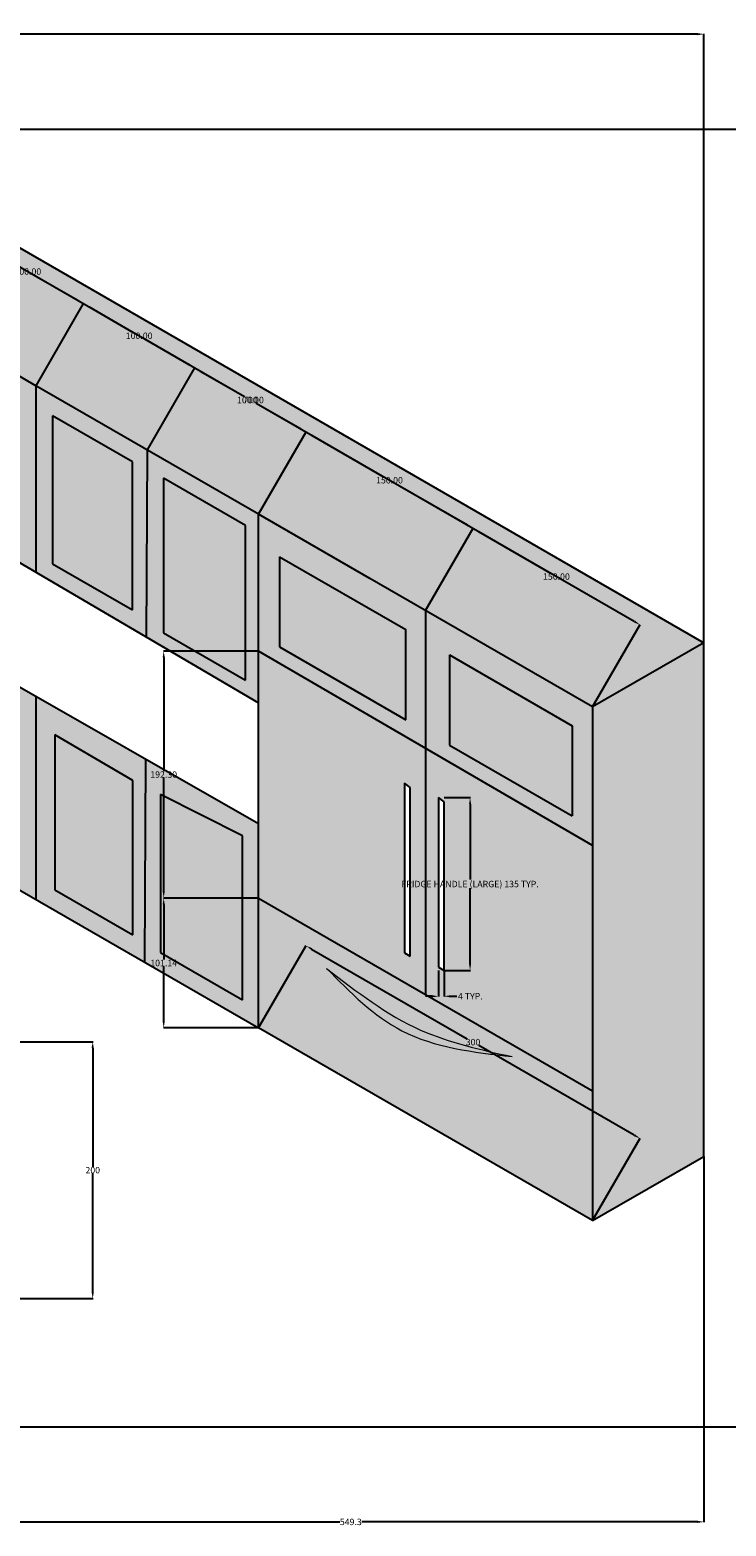
# Model space of a CAD drawing. Units: centimetres. Extents: x -744 to 1642, y 210 to 1375.
# Tile 4 of 8: x 288 to 830, y 210 to 1375. Entities that reach past the tile are written whole.
import ezdxf

# ---------------------------------------------------------------- set-up
doc = ezdxf.new("R2010")
doc.units = ezdxf.units.CM
doc.header["$MEASUREMENT"] = 0
for name, color, linetype, lineweight in [('A-ANNO-DIMS', 2, 'Continuous', 18), ('A-EQPM', 8, 'Continuous', 18), ('A-EQPM-PATT', 9, 'Continuous', 13), ('A-FURN', 7, 'Continuous', 25), ('A-FURN-PATT', 30, 'Continuous', 13), ('A-WALL-PATT', 61, 'Continuous', 13)]:
    doc.layers.add(name, color=color, linetype=linetype, lineweight=lineweight)
doc.styles.get("Standard").update_dxf_attribs({"font": 'arial.ttf'})
doc.dimstyles.get("Standard").update_dxf_attribs({"dimtxt": 5, "dimasz": 5, "dimexe": 0.18, "dimexo": 0.0625, "dimgap": 0.09, "dimtad": 0, "dimtih": 1, "dimtoh": 1, "dimdec": 0, "dimzin": 0, "dimdsep": 46, "dimtxsty": 'Standard', "dimcen": 0.09, "dimadec": 0, "dimazin": 0, "dimtfac": 1, "dimtdec": 0, "dimtofl": 0, "dimtmove": 0, "dimatfit": 3, "dimfxl": 1, "dimtolj": 1, "dimtzin": 0, "dimarcsym": 0})

# ---------------------------------------------------------------- blocks, each defined once
blk = doc.blocks.new('HANDLE-FRIDGE-LARGE')
for p, q in [((0, 134.6), (0, 2.5)), ((4.4, 131.3), (0, 134.6)), ((4.4, 0), (4.4, 131.3)), ((0, 2.5), (4.4, 0))]:
    blk.add_line(p, q)
blk = doc.blocks.new('*D3')
at = {"layer": 'A-ANNO-DIMS', "color": 0, "lineweight": -2, "transparency": 16777216}
for p, q in [((610.3, 777.6), (630.6, 777.6)), ((630.4, 772.6), (630.4, 713.7)), ((630.4, 648), (630.4, 707)), ((610.3, 643), (630.6, 643))]:
    blk.add_line(p, q, dxfattribs=at)
at = {"layer": 'A-ANNO-DIMS', "color": 0, "transparency": 16777216}
for points in [[(629.6, 772.6), (631.2, 772.6), (630.4, 777.6)], [(629.6, 648), (631.2, 648), (630.4, 643)]]:
    blk.add_solid(points, dxfattribs=at)
at = {"layer": 'Defpoints', "color": 0, "transparency": 16777216}
for p in [(610.2, 777.6), (630.4, 777.6), (610.2, 643)]:
    blk.add_point(p, dxfattribs=at)
at = {"layer": 'A-ANNO-DIMS', "color": 0, "transparency": 16777216, "insert": (630.4, 710.3), "char_height": 5, "attachment_point": 5}
blk.add_mtext('\\A1;FRIDGE HANDLE (LARGE) 135 TYP.', dxfattribs=at)
blk = doc.blocks.new('*D4')
at = {"layer": 'A-ANNO-DIMS', "color": 0, "lineweight": -2, "transparency": 16777216}
for p, q in [((605.8, 643), (605.8, 622.7)), ((610.2, 643), (610.2, 622.7)), ((600.8, 622.9), (595.8, 622.9)), ((615.2, 622.9), (620.2, 622.9))]:
    blk.add_line(p, q, dxfattribs=at)
at = {"layer": 'A-ANNO-DIMS', "color": 0, "transparency": 16777216}
for points in [[(600.8, 623.7), (600.8, 622), (605.8, 622.9)], [(615.2, 623.7), (615.2, 622), (610.2, 622.9)]]:
    blk.add_solid(points, dxfattribs=at)
at = {"layer": 'Defpoints', "color": 0, "transparency": 16777216}
for p in [(605.8, 643), (610.2, 643), (610.2, 622.9)]:
    blk.add_point(p, dxfattribs=at)
at = {"layer": 'A-ANNO-DIMS', "color": 0, "transparency": 16777216, "insert": (630.6, 622.9), "char_height": 5, "attachment_point": 5}
blk.add_mtext('\\A1;4 TYP.', dxfattribs=at)
blk = doc.blocks.new('*D7')
at = {"layer": 'A-ANNO-DIMS', "color": 0, "lineweight": -2, "transparency": 16777216}
for p, q in [((-660, 848.3), (-660, 1372.3)), ((-655, 1372.1), (65.9, 1372.1)), ((807.3, 1372.1), (86.3, 1372.1)), ((812.3, 898.3), (812.3, 1372.3))]:
    blk.add_line(p, q, dxfattribs=at)
at = {"layer": 'A-ANNO-DIMS', "color": 0, "transparency": 16777216}
for points in [[(-655, 1372.9), (-655, 1371.2), (-660, 1372.1)], [(807.3, 1372.9), (807.3, 1371.2), (812.3, 1372.1)]]:
    blk.add_solid(points, dxfattribs=at)
at = {"layer": 'Defpoints', "color": 0, "transparency": 16777216}
for p in [(812.3, 1372.1), (812.3, 898.2), (-660, 848.2)]:
    blk.add_point(p, dxfattribs=at)
at = {"layer": 'A-ANNO-DIMS', "color": 0, "transparency": 16777216, "insert": (76.1, 1372.1), "char_height": 5, "attachment_point": 5}
blk.add_mtext('\\A1;1472.2', dxfattribs=at)
blk = doc.blocks.new('*D9')
at = {"layer": 'A-ANNO-DIMS', "color": 0, "lineweight": -2, "transparency": 16777216}
for p, q in [((812.3, 498.2), (812.3, 213.5)), ((262.9, 387.4), (262.9, 213.5)), ((267.9, 213.6), (529.1, 213.6)), ((807.3, 213.6), (546.1, 213.6))]:
    blk.add_line(p, q, dxfattribs=at)
at = {"layer": 'A-ANNO-DIMS', "color": 0, "transparency": 16777216}
for points in [[(267.9, 214.5), (267.9, 212.8), (262.9, 213.6)], [(807.3, 214.5), (807.3, 212.8), (812.3, 213.6)]]:
    blk.add_solid(points, dxfattribs=at)
at = {"layer": 'Defpoints', "color": 0, "transparency": 16777216}
for p in [(812.3, 498.2), (262.9, 387.5), (812.3, 213.6)]:
    blk.add_point(p, dxfattribs=at)
at = {"layer": 'A-ANNO-DIMS', "color": 0, "transparency": 16777216, "insert": (537.6, 213.6), "char_height": 5, "attachment_point": 5}
blk.add_mtext('\\A1;549.3', dxfattribs=at)
blk = doc.blocks.new('*D10')
at = {"layer": 'A-ANNO-DIMS', "color": 0, "lineweight": -2, "transparency": 16777216}
for p, q in [((119.5, 1298.2), (886.3, 1298.2)), ((886.1, 1293.2), (886.1, 795.5)), ((886.1, 292.5), (886.1, 790.2)), ((89.8, 287.5), (886.3, 287.5))]:
    blk.add_line(p, q, dxfattribs=at)
at = {"layer": 'A-ANNO-DIMS', "color": 0, "transparency": 16777216}
for points in [[(885.3, 1293.2), (886.9, 1293.2), (886.1, 1298.2)], [(885.3, 292.5), (886.9, 292.5), (886.1, 287.5)]]:
    blk.add_solid(points, dxfattribs=at)
at = {"layer": 'Defpoints', "color": 0, "transparency": 16777216}
for p in [(119.4, 1298.2), (886.1, 1298.2), (89.7, 287.5)]:
    blk.add_point(p, dxfattribs=at)
at = {"layer": 'A-ANNO-DIMS', "color": 0, "transparency": 16777216, "insert": (886.1, 792.9), "char_height": 5, "attachment_point": 5}
blk.add_mtext('\\A1;1010.7', dxfattribs=at)
blk = doc.blocks.new('*D17')
at = {"layer": 'A-ANNO-DIMS', "color": 0, "lineweight": -2, "transparency": 16777216}
for p, q in [((119.5, 1198.3), (156.4, 1262.3)), ((160.7, 1259.7), (454.9, 1089.8)), ((758.2, 914.7), (464, 1084.5)), ((725.7, 848.3), (762.7, 912.3))]:
    blk.add_line(p, q, dxfattribs=at)
at = {"layer": 'A-ANNO-DIMS', "color": 0, "transparency": 16777216}
for points in [[(161.1, 1260.4), (160.3, 1259), (156.4, 1262.2)], [(758.7, 915.4), (757.8, 914), (762.6, 912.2)]]:
    blk.add_solid(points, dxfattribs=at)
at = {"layer": 'Defpoints', "color": 0, "transparency": 16777216}
for p in [(119.4, 1198.2), (762.6, 912.2), (725.7, 848.2)]:
    blk.add_point(p, dxfattribs=at)
at = {"layer": 'A-ANNO-DIMS', "color": 0, "transparency": 16777216, "insert": (459.5, 1087.2), "char_height": 5, "attachment_point": 5}
blk.add_mtext('\\A1;700', dxfattribs=at)
blk = doc.blocks.new('*D19')
at = {"layer": 'A-ANNO-DIMS', "color": 0, "lineweight": -2, "transparency": 16777216}
for p, q in [((465.9, 598.3), (502.9, 662.3)), ((507.1, 659.7), (628.1, 589.8)), ((758.2, 514.7), (637.3, 584.5)), ((725.7, 448.3), (762.7, 512.3))]:
    blk.add_line(p, q, dxfattribs=at)
at = {"layer": 'A-ANNO-DIMS', "color": 0, "transparency": 16777216}
for points in [[(507.5, 660.4), (506.7, 659), (502.8, 662.2)], [(758.7, 515.4), (757.8, 514), (762.6, 512.2)]]:
    blk.add_solid(points, dxfattribs=at)
at = {"layer": 'Defpoints', "color": 0, "transparency": 16777216}
for p in [(465.8, 598.2), (762.6, 512.2), (725.7, 448.2)]:
    blk.add_point(p, dxfattribs=at)
at = {"layer": 'A-ANNO-DIMS', "color": 0, "transparency": 16777216, "insert": (632.7, 587.2), "char_height": 5, "attachment_point": 5}
blk.add_mtext('\\A1;300', dxfattribs=at)
blk = doc.blocks.new('*D20')
at = {"layer": 'A-ANNO-DIMS', "color": 0, "lineweight": -2, "transparency": 16777216}
for p, q in [((465.8, 699.4), (391.8, 699.4)), ((392, 694.4), (392, 651.4)), ((392, 603.2), (392, 646.2)), ((465.8, 598.2), (391.8, 598.2))]:
    blk.add_line(p, q, dxfattribs=at)
at = {"layer": 'A-ANNO-DIMS', "color": 0, "transparency": 16777216}
for points in [[(391.2, 694.4), (392.8, 694.4), (392, 699.4)], [(391.2, 603.2), (392.8, 603.2), (392, 598.2)]]:
    blk.add_solid(points, dxfattribs=at)
at = {"layer": 'Defpoints', "color": 0, "transparency": 16777216}
for p in [(392, 699.4), (465.8, 699.4), (465.8, 598.2)]:
    blk.add_point(p, dxfattribs=at)
at = {"layer": 'A-ANNO-DIMS', "color": 0, "transparency": 16777216, "insert": (392, 648.8), "char_height": 5, "attachment_point": 5}
blk.add_mtext('\\A1;101.14', dxfattribs=at)
blk = doc.blocks.new('*D25')
at = {"layer": 'A-ANNO-DIMS', "color": 0, "lineweight": -2, "transparency": 16777216}
for p, q in [((263, 587.5), (337, 587.5)), ((336.8, 582.5), (336.8, 490.1)), ((336.8, 392.5), (336.8, 484.8)), ((263, 387.5), (337, 387.5))]:
    blk.add_line(p, q, dxfattribs=at)
at = {"layer": 'A-ANNO-DIMS', "color": 0, "transparency": 16777216}
for points in [[(335.9, 582.5), (337.6, 582.5), (336.8, 587.5)], [(335.9, 392.5), (337.6, 392.5), (336.8, 387.5)]]:
    blk.add_solid(points, dxfattribs=at)
at = {"layer": 'Defpoints', "color": 0, "transparency": 16777216}
for p in [(262.9, 587.5), (262.9, 387.5), (336.8, 387.5)]:
    blk.add_point(p, dxfattribs=at)
at = {"layer": 'A-ANNO-DIMS', "color": 0, "transparency": 16777216, "insert": (336.8, 487.5), "char_height": 5, "attachment_point": 5}
blk.add_mtext('\\A1;200', dxfattribs=at)
blk = doc.blocks.new('*D53')
at = {"layer": 'A-ANNO-DIMS', "color": 0, "lineweight": -2, "transparency": 16777216}
for p, q in [((206.1, 1148.3), (243.1, 1212.3)), ((247.3, 1209.7), (281.7, 1189.8)), ((325.2, 1164.7), (290.8, 1184.5)), ((292.7, 1098.3), (329.7, 1162.3))]:
    blk.add_line(p, q, dxfattribs=at)
at = {"layer": 'A-ANNO-DIMS', "color": 0, "transparency": 16777216}
for points in [[(247.7, 1210.4), (246.9, 1209), (243, 1212.2)], [(325.7, 1165.4), (324.8, 1164), (329.6, 1162.2)]]:
    blk.add_solid(points, dxfattribs=at)
at = {"layer": 'Defpoints', "color": 0, "transparency": 16777216}
for p in [(329.6, 1162.2), (206, 1148.2), (292.6, 1098.2)]:
    blk.add_point(p, dxfattribs=at)
at = {"layer": 'A-ANNO-DIMS', "color": 0, "transparency": 16777216, "insert": (286.3, 1187.2), "char_height": 5, "attachment_point": 5}
blk.add_mtext('\\A1;100.00', dxfattribs=at)
blk = doc.blocks.new('*D54')
at = {"layer": 'A-ANNO-DIMS', "color": 0, "lineweight": -2, "transparency": 16777216}
for p, q in [((292.7, 1098.3), (329.7, 1162.3)), ((333.9, 1159.7), (368.3, 1139.8)), ((411.8, 1114.7), (377.4, 1134.5)), ((379.3, 1048.3), (416.3, 1112.3))]:
    blk.add_line(p, q, dxfattribs=at)
at = {"layer": 'A-ANNO-DIMS', "color": 0, "transparency": 16777216}
for points in [[(334.3, 1160.4), (333.5, 1159), (329.6, 1162.2)], [(412.3, 1115.4), (411.4, 1114), (416.2, 1112.2)]]:
    blk.add_solid(points, dxfattribs=at)
at = {"layer": 'Defpoints', "color": 0, "transparency": 16777216}
for p in [(416.2, 1112.2), (292.6, 1098.2), (379.2, 1048.2)]:
    blk.add_point(p, dxfattribs=at)
at = {"layer": 'A-ANNO-DIMS', "color": 0, "transparency": 16777216, "insert": (372.9, 1137.2), "char_height": 5, "attachment_point": 5}
blk.add_mtext('\\A1;100.00', dxfattribs=at)
blk = doc.blocks.new('*D55')
at = {"layer": 'A-ANNO-DIMS', "color": 0, "lineweight": -2, "transparency": 16777216}
for p, q in [((379.3, 1048.3), (416.3, 1112.3)), ((420.5, 1109.7), (454.9, 1089.8)), ((498.4, 1064.7), (464, 1084.5)), ((465.9, 998.3), (502.9, 1062.3))]:
    blk.add_line(p, q, dxfattribs=at)
at = {"layer": 'A-ANNO-DIMS', "color": 0, "transparency": 16777216}
for points in [[(420.9, 1110.4), (420.1, 1109), (416.2, 1112.2)], [(498.9, 1065.4), (498, 1064), (502.8, 1062.2)]]:
    blk.add_solid(points, dxfattribs=at)
at = {"layer": 'Defpoints', "color": 0, "transparency": 16777216}
for p in [(502.8, 1062.2), (379.2, 1048.2), (465.8, 998.2)]:
    blk.add_point(p, dxfattribs=at)
at = {"layer": 'A-ANNO-DIMS', "color": 0, "transparency": 16777216, "insert": (459.5, 1087.2), "char_height": 5, "attachment_point": 5}
blk.add_mtext('\\A1;100.00', dxfattribs=at)
blk = doc.blocks.new('*D56')
at = {"layer": 'A-ANNO-DIMS', "color": 0, "lineweight": -2, "transparency": 16777216}
for p, q in [((465.9, 998.3), (502.9, 1062.3)), ((507.1, 1059.7), (563.1, 1027.3)), ((628.3, 989.7), (572.3, 1022)), ((595.8, 923.3), (632.8, 987.3))]:
    blk.add_line(p, q, dxfattribs=at)
at = {"layer": 'A-ANNO-DIMS', "color": 0, "transparency": 16777216}
for points in [[(507.5, 1060.4), (506.7, 1059), (502.8, 1062.2)], [(628.8, 990.4), (627.9, 989), (632.7, 987.2)]]:
    blk.add_solid(points, dxfattribs=at)
at = {"layer": 'Defpoints', "color": 0, "transparency": 16777216}
for p in [(465.8, 998.2), (632.7, 987.2), (595.7, 923.2)]:
    blk.add_point(p, dxfattribs=at)
at = {"layer": 'A-ANNO-DIMS', "color": 0, "transparency": 16777216, "insert": (567.7, 1024.7), "char_height": 5, "attachment_point": 5}
blk.add_mtext('\\A1;150.00', dxfattribs=at)
blk = doc.blocks.new('*D57')
at = {"layer": 'A-ANNO-DIMS', "color": 0, "lineweight": -2, "transparency": 16777216}
for p, q in [((595.8, 923.3), (632.8, 987.3)), ((637, 984.7), (693, 952.3)), ((758.2, 914.7), (702.2, 947)), ((725.7, 848.3), (762.7, 912.3))]:
    blk.add_line(p, q, dxfattribs=at)
at = {"layer": 'A-ANNO-DIMS', "color": 0, "transparency": 16777216}
for points in [[(637.4, 985.4), (636.6, 984), (632.7, 987.2)], [(758.7, 915.4), (757.8, 914), (762.6, 912.2)]]:
    blk.add_solid(points, dxfattribs=at)
at = {"layer": 'Defpoints', "color": 0, "transparency": 16777216}
for p in [(595.7, 923.2), (762.6, 912.2), (725.7, 848.2)]:
    blk.add_point(p, dxfattribs=at)
at = {"layer": 'A-ANNO-DIMS', "color": 0, "transparency": 16777216, "insert": (697.6, 949.7), "char_height": 5, "attachment_point": 5}
blk.add_mtext('\\A1;150.00', dxfattribs=at)
blk = doc.blocks.new('*D59')
at = {"layer": 'A-ANNO-DIMS', "color": 0, "lineweight": -2, "transparency": 16777216}
for p, q in [((465.8, 891.7), (391.8, 891.7)), ((392, 886.7), (392, 798.2)), ((392, 704.4), (392, 792.9)), ((465.8, 699.4), (391.8, 699.4))]:
    blk.add_line(p, q, dxfattribs=at)
at = {"layer": 'A-ANNO-DIMS', "color": 0, "transparency": 16777216}
for points in [[(391.2, 886.7), (392.8, 886.7), (392, 891.7)], [(391.2, 704.4), (392.8, 704.4), (392, 699.4)]]:
    blk.add_solid(points, dxfattribs=at)
at = {"layer": 'Defpoints', "color": 0, "transparency": 16777216}
for p in [(392, 891.7), (465.8, 891.7), (465.8, 699.4)]:
    blk.add_point(p, dxfattribs=at)
at = {"layer": 'A-ANNO-DIMS', "color": 0, "transparency": 16777216, "insert": (392, 795.5), "char_height": 5, "attachment_point": 5}
blk.add_mtext('\\A1;192.30', dxfattribs=at)

msp = doc.modelspace()

# ---------------------------------------------------------------- hatches: boundary and pattern name
at = {"layer": 'A-EQPM-PATT'}
h = msp.add_hatch(color=256, dxfattribs=at)
h.dxf.hatch_style = 1
h.paths.add_polyline_path([(-98.1787, 959.5025), (-124.4818, 991.1041), (-283.2822, 904.7538), (-283.2822, 903.5283), (-257.4428, 867.552)])
h.paths.add_polyline_path([(-283.2822, 903.5283), (-283.2822, 877.9161), (-257.4428, 862.9977), (-257.4428, 867.552)])
h.paths.add_polyline_path([(-98.1787, 953.5165), (-98.1787, 959.5025), (-257.4428, 867.552), (-257.4428, 862.9977), (-257.4428, 861.5653)])
h.paths.add_polyline_path([(595.7475, 816.0455), (465.8437, 891.6699), (465.8437, 699.3662), (595.7475, 624.3662)])
h.paths.add_polyline_path([(579.2833, 788.737), (583.6533, 785.4908), (583.6533, 654.1832), (579.2833, 656.7062)], flags=16)
h.paths.add_polyline_path([(725.6513, 740.4211), (595.7475, 816.0455), (595.7475, 624.3662), (725.6513, 549.3662)])
h.paths.add_polyline_path([(610.2064, 643.0466), (605.8363, 645.5696), (605.8363, 777.6004), (610.2064, 774.3542)], flags=16)
h.paths.add_polyline_path([(595.7475, 624.3662), (465.8437, 699.3662), (465.8437, 598.2308), (725.6513, 448.2308), (725.6513, 549.3662)])
at = {"layer": 'A-FURN-PATT'}
h = msp.add_hatch(color=256, dxfattribs=at)
h.dxf.hatch_style = 1
h.paths.add_polyline_path([(709.906, 763.421), (709.906, 833.5619), (614.425, 888.6879), (614.425, 818.5469)])
h.paths.add_polyline_path([(482.0889, 965.0922), (482.0889, 894.9512), (580.3491, 838.2207), (580.3491, 908.3616)])
h.paths.add_polyline_path([(455.661, 989.3482), (391.7403, 1026.2528), (391.7403, 905.908), (455.661, 869.0034)])
h.paths.add_polyline_path([(367.6025, 1038.9798), (305.4698, 1074.8522), (305.4698, 959.5913), (367.6025, 923.719)])
h.paths.add_polyline_path([(283.2252, 1090.8212), (213.1748, 1130.1519), (213.1748, 1010.3029), (283.2252, 969.8593)])
h.paths.add_polyline_path([(197.085, 1142.1995), (128.5906, 1179.2565), (128.5906, 1060.1567), (197.085, 1020.6114)])
h.paths.add_polyline_path([(111.6616, 1060.697), (111.6616, 1182.612), (67.1993, 1156.9417), (67.1993, 1033.9561)])
h.paths.add_polyline_path([(51.1364, 1025.5999), (51.1364, 1146.3882), (8.133, 1121.5602), (10.63, 1002.2135)])
h.paths.add_polyline_path([(-7.1228, 994.0363), (-7.1228, 1112.7639), (-46.1416, 1090.2363), (-45.0502, 972.1389)])
h.paths.add_polyline_path([(-62.5525, 1080.1953), (-112.7586, 1051.2088), (-111.3243, 975.2962), (-98.1787, 959.5025), (-98.1787, 953.5165), (-110.7754, 946.2438), (-110.5757, 935.6761), (-62.5525, 963.4023)])
h.paths.add_polyline_path([(-131.9167, 1043.3731), (-194.3022, 1007.3548), (-194.3022, 960.6093), (-131.9167, 994.0283)])
h.paths.add_polyline_path([(-210.3768, 1001.0803), (-272.1227, 965.4313), (-272.1227, 916.524), (-210.3442, 952.1919)])
h.paths.add_polyline_path([(-295.3923, 940.164), (-352.6194, 907.1238), (-352.6194, 798.1578), (-299.691, 828.716), (-295.3923, 831.1979)])
h.paths.add_polyline_path([(-373.8641, 892.8311), (-430.554, 860.1012), (-428.9419, 756.8396), (-373.8641, 788.6388)])
h.paths.add_polyline_path([(-449.1461, 850.3626), (-500.1893, 820.8928), (-498.1887, 714.0073), (-449.1461, 742.322)])
h.paths.add_polyline_path([(-517.3336, 813.4139), (-562.861, 787.1286), (-563.3952, 675.4493), (-517.3336, 702.043)])
h.paths.add_polyline_path([(-518.4603, 570.0519), (-562.9383, 544.3726), (-563.4408, 418.3375), (-518.4603, 444.307)])
h.paths.add_polyline_path([(-371.5223, 654.8866), (-429.2034, 621.5845), (-429.2034, 495.8395), (-371.5223, 529.1417)])
h.paths.add_polyline_path([(-448.7547, 610.2965), (-500.7971, 580.2498), (-501.5895, 454.0473), (-449.5067, 484.1173)])
h.paths.add_polyline_path([(-351.4436, 666.4791), (-351.4436, 540.7341), (-295.2328, 573.1874), (-295.2328, 698.9324)])
h.paths.add_polyline_path([(-256.6887, 595.4409), (-256.6887, 687.4813), (-215.6652, 711.1662), (-215.6652, 744.8707), (-268.9239, 714.1219), (-268.9239, 588.3769)])
h.paths.add_polyline_path([(-193.7313, 723.8298), (-132.6965, 759.0682), (-132.6965, 792.7727), (-193.7313, 757.5343)])
h.paths.add_polyline_path([(-114.2, 769.7472), (-83.4836, 787.4813), (-73.2438, 781.5694), (-73.2438, 827.0978), (-114.2, 803.4517)])
h.paths.add_polyline_path([(-53.2271, 770.0128), (-7.0224, 743.3364), (-7.0224, 865.3308), (-53.2271, 838.6544)])
h.paths.add_polyline_path([(8.89, 748.7728), (52.5303, 773.9686), (52.5303, 899.7135), (8.89, 874.5177)])
h.paths.add_polyline_path([(68.067, 782.9387), (108.041, 806.0177), (108.041, 931.7626), (68.067, 908.6836)])
h.paths.add_polyline_path([(130.3442, 802.4419), (196.727, 764.1157), (196.727, 896.2228), (130.3442, 934.5489), (130.3442, 927.6391)])
h.paths.add_polyline_path([(220.7637, 875.3463), (220.7637, 755.5756), (282.3763, 720.0036), (282.3763, 835.7573), (282.3763, 840.4873)])
h.paths.add_polyline_path([(307.3754, 826.3434), (307.3754, 705.693), (368.1078, 670.6291), (368.1078, 790.9456)])
h.paths.add_polyline_path([(389.5829, 779.9795), (389.5829, 656.983), (453.252, 620.2237), (453.252, 747.8082)])
at = {"layer": 'A-WALL-PATT'}
h = msp.add_hatch(color=256, dxfattribs=at)
h.dxf.hatch_style = 1
h.paths.add_polyline_path([(-226.9766, 998.2308), (119.4335, 1198.2308), (292.6386, 1098.2308), (465.8437, 998.2308), (552.4462, 948.2308), (725.6513, 848.2308), (812.2538, 898.2308), (119.4335, 1298.2308), (-659.9893, 848.2308), (-573.3868, 798.2308)])
h.paths.add_polyline_path([(-573.3868, 798.2308), (-659.9893, 848.2308), (-659.9893, 448.2308), (-573.3868, 398.2308)])
h.paths.add_polyline_path([(-507.2972, 836.3877), (-573.3868, 798.2308), (-573.3868, 659.7809), (-507.2972, 697.4412)])
h.paths.add_polyline_path([(-562.861, 787.1286), (-517.3336, 813.4139), (-517.3336, 702.043), (-563.3952, 675.4493)], flags=16)
h.paths.add_polyline_path([(-441.2075, 735.1015), (-441.2075, 874.5446), (-507.2972, 836.3877), (-507.2972, 697.4412)])
h.paths.add_polyline_path([(-500.1893, 820.8928), (-449.1461, 850.3626), (-449.1461, 742.322), (-498.1887, 714.0073)], flags=16)
h.paths.add_polyline_path([(-362.2449, 780.0973), (-362.2449, 920.1337), (-441.2075, 874.5446), (-441.2075, 735.1015)])
h.paths.add_polyline_path([(-430.554, 860.1012), (-373.8641, 892.8311), (-373.8641, 788.6388), (-428.9419, 756.8396)], flags=16)
h.paths.add_polyline_path([(-283.2822, 825.0931), (-283.2822, 965.7228), (-362.2449, 920.1337), (-362.2449, 780.0973)])
h.paths.add_polyline_path([(-352.6194, 798.1578), (-352.6194, 907.1238), (-295.3923, 940.164), (-295.3923, 831.1979), (-299.691, 828.716)], flags=16)
h.paths.add_polyline_path([(-203.882, 947.929), (-203.5655, 1011.7473), (-226.9766, 998.2308), (-283.2822, 965.7228), (-283.2822, 904.7538)], flags=17)
h.paths.add_polyline_path([(-272.1227, 965.4313), (-210.3768, 1001.0803), (-210.3442, 952.1919), (-272.1227, 916.524)], flags=16)
h.paths.add_polyline_path([(-123.8488, 991.4483), (-123.8488, 1057.7717), (-203.5655, 1011.7473), (-203.882, 947.929)], flags=17)
h.paths.add_polyline_path([(-194.3022, 1007.3548), (-131.9167, 1043.3731), (-131.9167, 994.0283), (-194.3022, 960.6093)], flags=16)
h.paths.add_polyline_path([(-112.7586, 1051.2088), (-62.5525, 1080.1953), (-62.5525, 963.4023), (-110.5757, 935.6761), (-110.7754, 946.2438), (-123.8488, 938.6959), (-123.8488, 915.9442), (-53.7716, 955.8768), (-53.7716, 1098.2308), (-123.8488, 1057.7717), (-123.8488, 991.4483), (-123.8488, 990.3436), (-111.3243, 975.2962)], flags=17)
h.paths.add_polyline_path([(1.2011, 1129.9693), (-53.7716, 1098.2308), (-53.7716, 955.8768), (1.4435, 987.3403)], flags=17)
h.paths.add_polyline_path([(-46.1416, 1090.2363), (-7.1228, 1112.7639), (-7.1228, 994.0363), (-45.0502, 972.1389)], flags=16)
h.paths.add_polyline_path([(60.3173, 1164.1001), (1.2011, 1129.9693), (1.4435, 987.3403), (60.3173, 1020.8888)], flags=17)
h.paths.add_polyline_path([(8.133, 1121.5602), (51.1364, 1146.3882), (51.1364, 1025.5999), (10.63, 1002.2135)], flags=16)
h.paths.add_polyline_path([(119.4335, 1054.5754), (119.4335, 1198.2308), (60.3173, 1164.1001), (60.3173, 1020.8888)], flags=17)
h.paths.add_polyline_path([(67.1993, 1156.9417), (111.6616, 1182.612), (111.6616, 1060.697), (67.1993, 1033.9561)], flags=16)
h.paths.add_polyline_path([(206.0361, 1148.2308), (119.4335, 1198.2308), (119.4335, 1054.5754), (206.0361, 1003.7675)], flags=17)
h.paths.add_polyline_path([(128.5906, 1179.2565), (197.085, 1142.1995), (197.085, 1020.6114), (128.5906, 1060.1567)], flags=16)
h.paths.add_polyline_path([(206.0361, 1148.2308), (206.0361, 1003.7675), (292.6386, 952.9596), (292.6386, 1098.2308)], flags=17)
h.paths.add_polyline_path([(213.1748, 1130.1519), (283.2252, 1090.8212), (283.2252, 969.8593), (213.1748, 1010.3029)], flags=16)
h.paths.add_polyline_path([(292.6386, 1098.2308), (292.6386, 952.9596), (378.4066, 902.6412), (379.2411, 1048.2308)], flags=17)
h.paths.add_polyline_path([(305.4698, 1074.8522), (367.6025, 1038.9798), (367.6025, 923.719), (305.4698, 959.5913)], flags=16)
h.paths.add_polyline_path([(379.2411, 1048.2308), (378.4066, 902.6412), (465.8437, 851.3437), (465.8437, 998.2308)], flags=17)
h.paths.add_polyline_path([(391.7403, 1026.2528), (455.661, 989.3482), (455.661, 869.0034), (391.7403, 905.908)], flags=16)
h.paths.add_polyline_path([(552.4462, 948.2308), (465.8437, 998.2308), (465.8437, 891.6699), (595.7475, 816.0455), (595.7475, 923.2308)], flags=17)
h.paths.add_polyline_path([(482.0889, 965.0922), (580.3491, 908.3616), (580.3491, 838.2207), (482.0889, 894.9512)], flags=16)
h.paths.add_polyline_path([(595.7475, 923.2308), (595.7475, 816.0455), (725.6513, 740.4211), (725.6513, 848.2308)])
h.paths.add_polyline_path([(614.425, 888.6879), (709.906, 833.5619), (709.906, 763.421), (614.425, 818.5469)], flags=16)
h.paths.add_polyline_path([(812.2538, 898.2308), (725.6513, 848.2308), (725.6513, 740.4211), (725.6513, 448.2308), (812.2538, 498.2308)])
h.paths.add_polyline_path([(465.8437, 757.085), (377.8609, 807.4399), (376.9558, 649.5503), (465.8437, 598.2308)])
h.paths.add_polyline_path([(389.5829, 779.9795), (453.252, 747.8082), (453.252, 620.2237), (389.5829, 656.983)], flags=16)
h.paths.add_polyline_path([(377.8609, 807.4399), (292.6386, 856.215), (292.6386, 698.2308), (376.9558, 649.5503)])
h.paths.add_polyline_path([(368.1078, 670.6291), (307.3754, 705.693), (307.3754, 826.3434), (368.1078, 790.9456)], flags=16)
h.paths.add_polyline_path([(292.6386, 856.215), (206.0361, 905.7799), (206.0361, 748.2308), (292.6386, 698.2308)])
h.paths.add_polyline_path([(282.3763, 720.0036), (220.7637, 755.5756), (220.7637, 875.3463), (282.3763, 840.4873), (282.3763, 835.7573)], flags=16)
h.paths.add_polyline_path([(206.0361, 905.7799), (119.4335, 955.3449), (119.4335, 798.2308), (206.0361, 748.2308)])
h.paths.add_polyline_path([(196.727, 764.1157), (130.3442, 802.4419), (130.3442, 927.6391), (130.3442, 934.5489), (196.727, 896.2228)], flags=16)
h.paths.add_polyline_path([(119.4335, 955.3449), (60.5235, 921.3332), (60.5235, 764.2191), (119.4335, 798.2308)])
h.paths.add_polyline_path([(108.041, 806.0177), (68.067, 782.9387), (68.067, 908.6836), (108.041, 931.7626)], flags=16)
h.paths.add_polyline_path([(60.5235, 764.2191), (60.5235, 921.3332), (1.6135, 887.3215), (1.867, 738.2042), (3.1189, 737.4813), (8.6656, 734.279)])
h.paths.add_polyline_path([(8.89, 748.7728), (8.89, 874.5177), (52.5303, 899.7135), (52.5303, 773.9686)], flags=16)
h.paths.add_polyline_path([(1.6135, 887.3215), (-61.1176, 851.1036), (-61.1176, 774.5683), (-53.2271, 770.0128), (-53.2271, 838.6544), (-7.0224, 865.3308), (-7.0224, 743.3364), (1.867, 738.2042)])
h.paths.add_polyline_path([(-61.1176, 851.1036), (-123.8488, 814.8858), (-123.8488, 764.1765), (-114.2, 769.7472), (-114.2, 803.4517), (-73.2438, 827.0978), (-73.2438, 781.5694), (-61.1176, 774.5683)])
h.paths.add_polyline_path([(-132.6965, 792.7727), (-132.6965, 759.0682), (-123.8488, 764.1765), (-123.8488, 814.8858), (-203.5655, 768.8613), (-203.5655, 718.152), (-193.7313, 723.8298), (-193.7313, 757.5343)])
h.paths.add_polyline_path([(-203.5655, 768.8613), (-283.2822, 722.8369), (-283.2822, 565.7228), (-256.6887, 581.0766), (-256.6887, 595.4409), (-268.9239, 588.3769), (-268.9239, 714.1219), (-215.6652, 744.8707), (-215.6652, 711.1662), (-203.5655, 718.152)])
h.paths.add_polyline_path([(-283.2822, 722.8369), (-362.2449, 677.2477), (-362.2449, 520.1337), (-283.2822, 565.7228)])
h.paths.add_polyline_path([(-295.2328, 573.1874), (-351.4436, 540.7341), (-351.4436, 666.4791), (-295.2328, 698.9324)], flags=16)
h.paths.add_polyline_path([(-362.2449, 677.2477), (-441.2075, 631.6586), (-441.2075, 474.5446), (-362.2449, 520.1337)])
h.paths.add_polyline_path([(-371.5223, 529.1417), (-429.2034, 495.8395), (-429.2034, 621.5845), (-371.5223, 654.8866)], flags=16)
h.paths.add_polyline_path([(-441.2075, 631.6586), (-507.2972, 593.5018), (-507.2972, 436.3877), (-441.2075, 474.5446)])
h.paths.add_polyline_path([(-448.7547, 610.2965), (-449.5067, 484.1173), (-501.5895, 454.0473), (-500.7971, 580.2498)], flags=16)
h.paths.add_polyline_path([(-507.2972, 593.5018), (-573.3868, 555.3449), (-573.3868, 398.2308), (-507.2972, 436.3877)])
h.paths.add_polyline_path([(-518.4603, 570.0519), (-518.4603, 444.307), (-563.4408, 418.3375), (-562.9383, 544.3726)], flags=16)
h.paths.add_polyline_path([(-118.6694, 598.5582), (-123.6694, 601.445), (-123.6694, 488.0238), (-118.6694, 485.1326)], flags=17)
h.paths.add_polyline_path([(-113.6694, 595.6715), (-118.6694, 598.5582), (-118.6694, 485.1326), (-113.6694, 482.2413)], flags=17)
h.paths.add_polyline_path([(-12.0425, 536.9972), (-17.0425, 539.8839), (-17.0425, 426.3672), (-12.0425, 423.4759)], flags=17)
h.paths.add_polyline_path([(-17.0425, 539.8839), (-22.0425, 542.7707), (-22.0425, 429.2584), (-17.0425, 426.3672)], flags=17)
h.paths.add_polyline_path([(-256.6887, 687.4813), (-256.6887, 487.4813), (-248.6887, 482.8625), (-248.6887, 673.6249), (81.7215, 482.8625), (81.7215, 292.1001), (89.7215, 287.4813), (89.7215, 487.4813)])
h.paths.add_polyline_path([(-196.8604, 530.3463), (-196.7272, 512.8625), (81.7215, 352.1001), (81.7215, 369.2572)], flags=17)

# ---------------------------------------------------------------- linework, layer by layer
at = {"layer": 'A-EQPM'}
for points, knots in [([(518.7785, 644.5639), (542.1869, 626.4466), (585.4359, 592.9733), (638.7101, 581.2683), (663.1498, 575.8985)], [0, 0, 0, 0, 87.488642647, 161.642932127, 161.642932127, 161.642932127, 161.642932127]), ([(518.7785, 644.5639), (537.124, 625.9721), (576.6962, 585.8686), (632.9663, 579.3794), (663.1498, 575.8985)], [0, 0, 0, 0, 76.118982026, 164.192735849, 164.192735849, 164.192735849, 164.192735849])]:
    msp.add_open_spline(points, degree=3, knots=knots, dxfattribs=at)
at = {"layer": 'A-FURN'}
for p, q in [((119.4335, 1298.2308), (812.2538, 898.2308)), ((292.6386, 1098.2308), (119.4335, 1198.2308)), ((465.8437, 998.2308), (292.6386, 1098.2308)), ((292.6386, 1098.2308), (292.6386, 952.9596)), ((305.4698, 1074.8522), (305.4698, 959.5913)), ((367.6025, 1038.9798), (305.4698, 1074.8522)), ((119.4335, 1054.5754), (465.8437, 851.3437)), ((367.6025, 923.719), (367.6025, 1038.9798)), ((379.2411, 1048.2308), (378.4066, 902.6412)), ((391.7403, 1026.2528), (391.7403, 905.908)), ((455.661, 989.3482), (391.7403, 1026.2528)), ((552.4462, 948.2308), (465.8437, 998.2308)), ((465.8437, 598.2308), (465.8437, 998.2308)), ((455.661, 869.0034), (455.661, 989.3482)), ((465.8437, 757.085), (119.4335, 955.3449)), ((305.4698, 959.5913), (367.6025, 923.719)), ((482.0889, 965.0922), (482.0889, 894.9512)), ((482.0889, 965.0922), (580.3491, 908.3616)), ((725.6513, 848.2308), (552.4462, 948.2308)), ((595.7475, 923.2308), (595.7475, 624.3662)), ((391.7403, 905.908), (455.661, 869.0034)), ((580.3491, 838.2207), (580.3491, 908.3616)), ((812.2538, 898.2308), (725.6513, 848.2308)), ((812.2538, 498.2308), (812.2538, 898.2308)), ((725.6513, 740.4211), (465.8437, 891.6699)), ((482.0889, 894.9512), (580.3491, 838.2207)), ((614.425, 888.6879), (709.906, 833.5619)), ((614.425, 888.6879), (614.425, 818.5469)), ((292.6386, 856.215), (292.6386, 698.2308)), ((725.6513, 848.2308), (725.6513, 448.2308)), ((709.906, 833.5619), (709.906, 763.421)), ((307.3754, 826.3434), (307.3754, 705.693)), ((368.1078, 790.9456), (307.3754, 826.3434)), ((614.425, 818.5469), (709.906, 763.421)), ((377.8609, 807.4399), (376.9558, 649.5503)), ((119.4335, 798.2308), (465.8437, 598.2308)), ((368.1078, 670.6291), (368.1078, 790.9456)), ((389.5829, 779.9795), (389.5829, 656.983)), ((453.252, 747.8082), (389.5829, 779.9795)), ((453.252, 620.2237), (453.252, 747.8082)), ((307.3754, 705.693), (368.1078, 670.6291)), ((465.8437, 699.3662), (725.6513, 549.3662)), ((389.5829, 656.983), (453.252, 620.2237)), ((725.6513, 448.2308), (465.8437, 598.2308)), ((725.6513, 448.2308), (812.2538, 498.2308))]:
    msp.add_line(p, q, dxfattribs=at)

# ---------------------------------------------------------------- block references
for p in [(579.283, 654.1836), (605.836, 643.047)]:
    msp.add_blockref('HANDLE-FRIDGE-LARGE', p, dxfattribs=at)

# ---------------------------------------------------------------- dimensions: what is measured, and where the dimension line sits
at = {"layer": 'A-ANNO-DIMS'}
for base, p1, p2, picture, middle in [((812.2538, 1372.0808), (-659.9893, 848.2308), (812.2538, 898.2308), '*D7', (76.1323, 1372.0808)), ((812.2538, 213.6313), (262.9266, 387.4813), (812.2538, 498.2308), '*D9', (537.5902, 213.6313))]:
    dim = msp.add_linear_dim(base=base, p1=p1, p2=p2, dimstyle='Standard', override={"dimdec": 1, "dimlfac": 1, "dimrnd": 0, "dimzin": 0, "dimdsep": 46, "dimlunit": 2}, dxfattribs=at)
    dim.commit()
    dim.dimension.update_dxf_attribs({"geometry": picture, "text_midpoint": middle})
for base, p1, p2, angle, override, picture, middle in [((886.1038, 1298.2308), (89.7215, 287.4813), (119.4335, 1298.2308), 90, {"dimdec": 1, "dimlfac": 1, "dimrnd": 0, "dimzin": 0, "dimdsep": 46, "dimlunit": 2}, '*D10', (886.1038, 792.8561)), ((762.5763, 912.1868), (119.4335, 1198.2308), (725.6513, 848.2308), 330, {"dimdec": 0, "dimlfac": 1, "dimrnd": 0, "dimzin": 0, "dimdsep": 46, "dimlunit": 2}, '*D17', (459.4674, 1087.1868)), ((329.5636, 1162.1868), (206.0361, 1148.2308), (292.6386, 1098.2308), 330, {"dimdec": 2, "dimlfac": 1, "dimrnd": 0, "dimzin": 0, "dimdsep": 46, "dimlunit": 2}, '*D53', (286.2623, 1187.1868)), ((416.1661, 1112.1868), (292.6386, 1098.2308), (379.2411, 1048.2308), 330, {"dimdec": 2, "dimlfac": 1, "dimrnd": 0, "dimzin": 0, "dimdsep": 46, "dimlunit": 2}, '*D54', (372.8649, 1137.1868)), ((502.7687, 1062.1868), (379.2411, 1048.2308), (465.8437, 998.2308), 330, {"dimdec": 2, "dimlfac": 1, "dimrnd": 0, "dimzin": 0, "dimdsep": 46, "dimlunit": 2}, '*D55', (459.4674, 1087.1868)), ((632.6725, 987.1868), (465.8437, 998.2308), (595.7475, 923.2308), 330, {"dimdec": 2, "dimlfac": 1, "dimrnd": 0, "dimzin": 0, "dimdsep": 46, "dimlunit": 2}, '*D56', (567.7206, 1024.6868)), ((762.5763, 912.1868), (595.7475, 923.2308), (725.6513, 848.2308), 330, {"dimdec": 2, "dimlfac": 1, "dimrnd": 0, "dimzin": 0, "dimdsep": 46, "dimlunit": 2}, '*D57', (697.6244, 949.6868)), ((391.9937, 891.6699), (465.8437, 699.3662), (465.8437, 891.6699), 90, {"dimdec": 2, "dimlfac": 1, "dimrnd": 0, "dimzin": 0, "dimdsep": 46, "dimlunit": 2}, '*D59', (391.9937, 795.518)), ((391.9937, 699.3662), (465.8437, 598.2308), (465.8437, 699.3662), 90, {"dimdec": 2, "dimlfac": 1, "dimrnd": 0, "dimzin": 0, "dimdsep": 46, "dimlunit": 2}, '*D20', (391.9937, 648.7985)), ((762.5763, 512.1868), (465.8437, 598.2308), (725.6513, 448.2308), 330, {"dimdec": 0, "dimlfac": 1, "dimrnd": 0, "dimzin": 0, "dimdsep": 46, "dimlunit": 2}, '*D19', (632.6725, 587.1868)), ((336.7766, 387.4813), (262.9266, 587.4813), (262.9266, 387.4813), 270, {"dimdec": 0, "dimlfac": 1, "dimrnd": 0, "dimzin": 0, "dimdsep": 46, "dimlunit": 2}, '*D25', (336.7766, 487.4813))]:
    dim = msp.add_linear_dim(base=base, p1=p1, p2=p2, angle=angle, dimstyle='Standard', override=override, dxfattribs=at)
    dim.commit()
    dim.dimension.update_dxf_attribs({"geometry": picture, "text_midpoint": middle})
dim = msp.add_linear_dim(base=(630.3895, 777.6004), p1=(610.2064, 643.0466), p2=(610.2064, 777.6004), angle=90, text='FRIDGE HANDLE (LARGE) <> TYP.', dimstyle='Standard', override={"dimdec": 0, "dimrnd": 0, "dimzin": 0, "dimlunit": 2}, dxfattribs=at)
dim.commit()
dim.dimension.update_dxf_attribs({"geometry": '*D3', "text_midpoint": (630.3895, 710.3235)})
dim = msp.add_linear_dim(base=(610.2064, 622.8635), p1=(605.8363, 643.0466), p2=(610.2064, 643.0466), text='<> TYP.', dimstyle='Standard', override={"dimdec": 0, "dimrnd": 0, "dimzin": 0, "dimlunit": 2}, dxfattribs=at)
dim.commit()
dim.dimension.update_dxf_attribs({"geometry": '*D4', "text_midpoint": (630.6238, 622.8635)})

doc.saveas('drawing.dxf')
